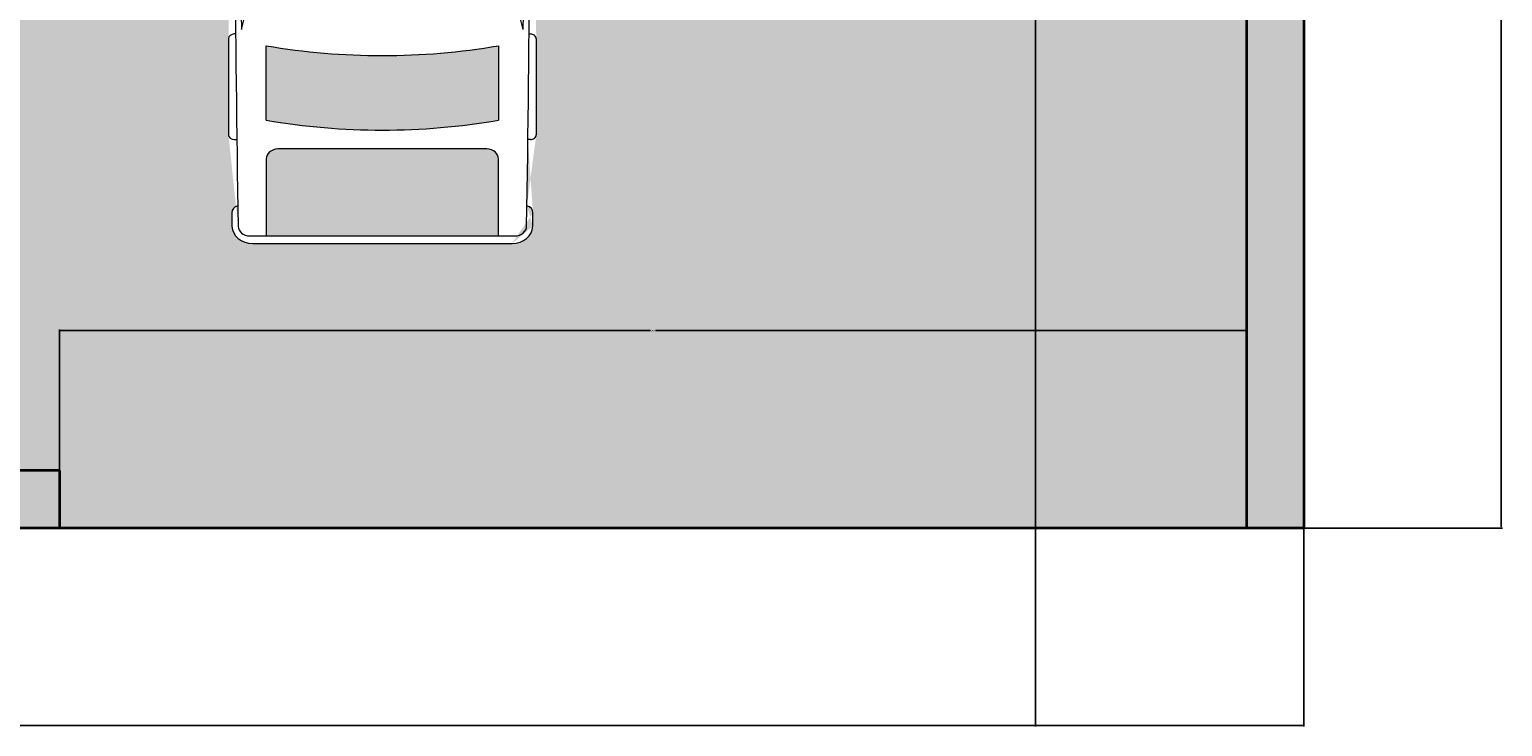
# Model space of a CAD drawing. Units: inches. Extents: x 2549 to 3108, y 1683 to 2362.
# Tile 4 of 30: x 2877 to 3108, y 1683 to 1793. Entities that reach past the tile are written whole.
import ezdxf

# ---------------------------------------------------------------- set-up
doc = ezdxf.new("R2010")
doc.units = ezdxf.units.IN
for name, color, linetype, lineweight in [('A-ANNO-DIMS', 2, 'Continuous', 18), ('C-PKNG-VEHI', 8, 'Continuous', 18), ('C-PROP', 7, 'Continuous', 35)]:
    doc.layers.add(name, color=color, linetype=linetype, lineweight=lineweight)
for name, color, linetype, lineweight, true_color in [('C-PKNG-VEHI-PATT', 251, 'Continuous', 13, 0x636466), ('C-PROP-PATT', 252, 'Continuous', 13, 0x939598), ('C-PVMT-PATT', 9, 'Continuous', 13, 0xc7c8ca)]:
    doc.layers.add(name, color=color, linetype=linetype, lineweight=lineweight, true_color=true_color)
doc.styles.get("Standard").update_dxf_attribs({"font": 'arial.ttf'})
doc.dimstyles.get("Standard").update_dxf_attribs({"dimtxt": 0.18, "dimasz": 0.18, "dimexe": 0.18, "dimexo": 0.0625, "dimgap": 0.09, "dimtad": 0, "dimtih": 1, "dimtoh": 1, "dimdec": 4, "dimzin": 0, "dimdsep": 46, "dimtxsty": 'Standard', "dimcen": 0.09, "dimadec": 0, "dimazin": 0, "dimtfac": 1, "dimtdec": 4, "dimtofl": 0, "dimtmove": 0, "dimatfit": 3, "dimfxl": 1, "dimtolj": 1, "dimtzin": 0, "dimarcsym": 0})

# ---------------------------------------------------------------- blocks, each defined once
blk = doc.blocks.new('*U11')
for p, q in [((21.10406751471477, 37.40863046792069), (21.10406751471477, 36.83230215753705)), ((46.55368679439944, 38.88847654282876), (22.35054758993934, 38.88847654282876)), ((47.80016686962392, 37.39011648242055), (47.80016686962392, 37.40863046792069)), ((135.4513231603356, 37.07354110333037), (135.4513231603356, 37.40863046792069)), ((136.6978032355602, 38.88847654282876), (160.90094244002, 38.88847654282867)), ((162.1474225152445, 37.40863046792049), (162.1474225152445, 36.77402019194128)), ((87.98532186932616, 31.87120872459877), (74.75900729854769, 35.92175679182955)), ((134.313356548143, 35.6043097713567), (119.2882629232503, 31.77757799177584)), ((70.0302824853563, 31.53613089391356), (86.40615155322342, 29.35124891408057)), ((186.4728846989705, -33.49860931502491), (186.4728846989718, 33.49860931502465)), ((188.3990091454065, -32.75868627757393), (188.3990091454077, 32.75868627757058)), ((138.4228833961707, 29.35124891408074), (157.2465674415997, 29.35124891408074)), ((164.515393597658, 26.39155676426461), (164.5153935976578, -26.39155676426503)), ((186.4728846989718, 29.35124891408083), (167.0083537481071, 29.35124891408083)), ((32.26591480791686, 11.62530558863241), (36.12873726252356, 17.16961494239206)), ((36.12873726252356, 17.16961494239206), (50.93891189819171, 17.16961494239206)), ((29.77279020470884, 9.505833383620029), (51.68362801571248, 9.505833383620029)), ((32.12291633764599, 9.505833383620029), (32.12291633764599, 11.15369945057711)), ((58.9167604809788, -10.77488335095668), (58.9167604809788, 10.77488335095617)), ((66.55009204259746, -10.5288681329018), (66.55009204259746, 10.52886813290129)), ((82.73706193978568, 8.496039918672748), (82.73706193978568, -8.49603991867258)), ((186.4728846989718, -10.5288681329018), (186.4728846989718, 10.52886813290129)), ((3.266462181856987, 6.128290093440767), (0.1022408397004821, 0.4060708604429806)), ((-4.43e-14, -2.558e-13), (51.68362801571248, -2.558e-13)), ((0.1022408397004821, -0.4060708604432933), (3.266462181856987, -6.128290093441194)), ((29.77279020470884, -9.50583338362054), (51.68362801571248, -9.50583338362054)), ((32.12291633764599, -9.50583338362054), (32.12291633764599, -11.15369945057762)), ((32.26591480791686, -11.62530558863292), (36.12873726252356, -17.16961494239257)), ((36.12873726252356, -17.16961494239257), (50.93891189819171, -17.16961494239257)), ((86.40615155322318, -29.35124891408145), (70.03028248535594, -31.53613089391442)), ((157.2465674415997, -29.35124891408117), (138.4228833961707, -29.35124891408126)), ((167.008353748107, -29.35124891408126), (186.4728846989707, -29.35124891408108)), ((87.98532186932607, -31.87120872459903), (74.7590072985476, -35.92175679182964)), ((134.3133565481428, -35.60430977135721), (119.2882629232503, -31.77757799177618)), ((21.10406751471477, -37.4086304679212), (21.10406751471477, -36.83230215753756)), ((135.4513231603355, -37.07354110333088), (135.4513231603355, -37.4086304679212)), ((162.1474225152445, -37.408630467921), (162.1474225152445, -36.77402019194179)), ((46.55368679439944, -38.88847654282927), (22.35054758993934, -38.88847654282927)), ((47.80016686962392, -37.39011648242107), (47.80016686962392, -37.4086304679212)), ((136.6978032355602, -38.88847654282927), (160.9009424400199, -38.88847654282918))]:
    blk.add_line(p, q)
for centre, major_axis, ratio, start_param, end_param in [((41.19115208863305, -490.8631038926156), (1.294e-13, 528.2339998381949), 0.8423038695439741, 0.0028100083536837, 0.0755983031096952), ((22.35054758993934, 37.40863046792072), (2.08e-14, -1.479846074908118), 0.842303869543976, 3.141592653589776, 4.712388980384677), ((64.48199294511879, -10555.61767587835), (1.907644e-10, 10593.02630634627), 0.842303869543847, -0.0133969486112073, 0.0027970409639888), ((46.55368679439944, 37.40863046792072), (2.2e-14, 1.479846074908118), 0.8423038695439758, -1.570796326794884, 1.73e-14), ((136.6978032355602, 37.40863046792072), (2.357e-13, -1.479846074908118), 0.842303869543976, 3.141592653589603, 4.712388980384554), ((160.90094244002, 37.40863046792052), (5.59e-14, 1.479846074908118), 0.842303869543976, -1.570796326794865, 4.44e-14), ((180.6280394947615, 35.8381667808375), (7.4e-14, 2.219769112362114), 0.8423038695439693, -0.0130174256259048, 1.249894140392862), ((64.48199294754608, -10556.35759891604), (1.349839377e-06, 10595.3130398087), 0.8423038681351469, -0.0133969484821159, -0.0130174254969711), ((183.9799245485216, 32.75868627756583), (8.56e-14, -5.246425615115243), 0.8423038695439737, 1.570796326795794, 3.128195704978164), ((266.0300214172791, -27.52442688366631), (1.966072e-10, 313.3077612809058), 0.8423038695435284, 1.367075990158062, 1.391760499156098), ((64.4819929449925, -10555.61767590795), (1.9177683e-09, -10591.54646030096), 0.8423038695482963, 3.133765086725325, 3.140440689641252), ((183.9799245485226, 33.49860931502124), (3e-16, -2.959692149816168), 0.8423038695439952, 1.570796326796048, 3.128195704978389), ((135.2911776514449, 5.387441675478555), (2.2715e-12, 81.77258453065997), 0.8423038695439563, 1.245306111696802, 1.507880129813836), ((95.78879860270445, -3666.353346297651), (1.949864e-10, -3698.236159209632), 0.8423038695446962, 3.134048706297306, 3.14409775411291), ((259.1750197310735, -27.52442688366614), (1.506617e-10, -305.3028914627677), 0.8423038695443789, 4.528606069860317, 4.561837674556238), ((37.47375371777758, -593.9621830607928), (6.21e-14, -623.32820996736), 0.8423038695439826, 3.09604606856106, 3.200911180495224), ((134.4003789125686, 5.387441675477674), (4.276e-13, -89.7774543484738), 0.84230386954398, 4.44948196380473, 4.652344057257214), ((149.595361812917, 2.799442537139299), (8.561e-13, -79.57966406425402), 0.842303869543983, 4.372215489277867, 4.640744122441986), ((17.08207736189386, -1.421e-13), (6.87e-14, 147.0179238898305), 0.8423038695439764, 4.511394369635731, 4.913383591133647), ((35.90576140732288, -1.421e-13), (6.87e-14, 147.0179238898305), 0.8423038695439764, 4.511394369635731, 4.913383591133647), ((167.0083537481071, 26.39155676426464), (1.394e-13, 2.959692149816236), 0.842303869543976, 5.55e-14, 1.57079632679492), ((-204.4946649195746, 52.39684969293512), (4.12053e-11, -250.9602162198571), 0.8423038695441164, 1.385369446298923, 1.434372047871027), ((13.03653510440275, 17.00972444508943), (1.2303e-12, 27.41599049210566), 0.8423038695439277, 4.435146050259648, 4.718221029521873), ((14.20086229321332, 17.00972444508943), (1.2303e-12, 27.41599049210566), 0.8423038695439277, 4.435146050259648, 4.718221029521873), ((50.7902773840875, 13.33772416300607), (6.340077547122382, -0.356608581037027), 0.6038335755719145, -1.39555193967809, 1.581314658479915), ((32.74615637525823, 11.15369945057713), (1.313e-13, 0.7399230374541176), 0.8423038695439091, 0.8797135699495516, 1.570796326795045), ((29.77279020470884, -46.66302566589627), (5.12e-14, 56.16885904951626), 0.842303869543976, 7e-16, 0.5903187773915901), ((0.6232400376122422, -1.421e-13), (1e-16, -0.7399230374541245), 0.842303869543842, 4.131459131953847, 5.293318828815531), ((29.77279020470884, 46.66302566589578), (4.004e-13, 56.16885904951626), 0.8423038695439734, 2.55127387619821, 3.141592653589801), ((-204.4946649195746, -52.39684969293552), (4.02945e-11, 250.9602162198562), 0.8423038695441192, -1.43437204787103, -1.385369446298926), ((32.74615637525823, -11.1536994505777), (1.3e-13, -0.7399230374541176), 0.8423038695439093, 4.712388980384541, 5.403471737230034), ((13.03653510440275, -17.00972444508983), (1.2568e-12, -27.41599049210552), 0.8423038695439318, 1.564964277657711, 1.848039256919935), ((14.20086229321332, -17.00972444508983), (1.2568e-12, -27.41599049210552), 0.8423038695439318, 1.564964277657711, 1.848039256919935), ((134.4003789125684, -5.387441675478584), (4.2949e-12, -89.77745434847827), 0.8423038695439354, -1.510751403667474, -1.307889310215002), ((135.2911776514465, -5.387441675480715), (3.2038e-12, -81.77258453066244), 0.8423038695439492, -1.50788012981387, -1.245306111696839), ((149.5953618129329, -2.799442537137565), (4.0897e-12, -79.57966406427697), 0.8423038695439419, -1.499151468852248, -1.230622835688196), ((259.1750197310694, 27.52442688365929), (1.08535e-11, 305.3028914629043), 0.8423038695439974, 1.721347632622872, 1.754579237318777), ((266.0300214172791, 27.52442688366566), (8.75241e-11, 313.3077612806533), 0.8423038695441819, 1.749832154434603, 1.774516663432659), ((37.47375371777847, 593.9621830607904), (1.1693e-12, -623.3282099673584), 0.8423038695439528, -0.0593185269054384, 0.0455465850287298), ((167.008353748107, -26.39155676426503), (1.02e-14, -2.959692149816192), 0.8423038695439885, 4.712388980384686, 6.283185307179581), ((95.78879860271888, 3666.35334629765), (1.637818e-10, -3698.236159209629), 0.8423038695447546, -0.0025051005232382, 0.007543947292366), ((183.9799245485216, -33.4986093150211), (9.3e-15, 2.959692149816141), 0.8423038695439732, 3.154989602201626, 4.71238898038339), ((183.9799245485177, -32.7586862775633), (2.428e-13, -5.246425615118353), 0.8423038695439808, 0.0133969486110846, 1.570796326792831), ((41.19115208863322, 490.8631038926152), (1.37757e-11, -528.2339998381949), 0.8423038695440652, -0.0755983031097181, -0.0028100083537155), ((64.48199294495228, 10555.61767590795), (6.117947e-10, 10593.02630637587), 0.8423038695458146, 3.138795612625926, 3.154989602201039), ((64.48199294503607, 10555.61767590793), (1.6049794e-09, -10591.54646030094), 0.8423038695397146, 0.0011519639481523, 0.0078275668641468), ((180.6280394947581, -35.83816678083949), (2.274e-13, -2.219769112363032), 0.8423038695439803, -1.249894138785958, 0.0130174256254374), ((22.35054758993934, -37.40863046792117), (2.2e-14, 1.479846074908118), 0.8423038695439758, 1.570796326794908, 3.14159265358981), ((46.55368679439944, -37.40863046792117), (2.08e-14, -1.479846074908118), 0.842303869543976, -1.69e-14, 1.570796326794884), ((136.6978032355602, -37.40863046792109), (1.56e-14, -1.479846074908162), 0.8423038695440105, -1.570796326794875, -1.27e-14), ((160.9009424400199, -37.408630467921), (1.969e-13, 1.479846074908162), 0.8423038695440109, 3.141592653589951, 4.712388980384771), ((64.48199294197605, 10556.3575989598), (9.365289701e-07, 10595.31303985772), 0.8423038705260315, 3.154610079306566, 3.154989602290631)]:
    blk.add_ellipse(centre, major_axis=major_axis, ratio=ratio, start_param=start_param, end_param=end_param)
at = {"extrusion": (0, 0, -1)}
blk.add_ellipse((50.7902773840875, -13.33772416300655), major_axis=(6.340077547122382, 0.3566085810370246), ratio=0.6038335755719145, start_param=-1.39555193967809, end_param=1.581314658479915, dxfattribs=at)
blk = doc.blocks.new('*D24')
at = {"layer": 'A-ANNO-DIMS', "color": 0, "lineweight": -2, "transparency": 16777216}
for p, q in [((2596.642666000001, 1714.461244), (2596.642666000001, 1683.443744)), ((3076.642666000001, 1714.461244), (3076.642666000001, 1683.443744)), ((2596.822666, 1683.623744), (2836.350503653479, 1683.623744)), ((3076.462666000001, 1683.623744), (2836.934828346521, 1683.623744))]:
    blk.add_line(p, q, dxfattribs=at)
at = {"layer": 'A-ANNO-DIMS', "color": 0, "transparency": 16777216}
for points in [[(2596.822666, 1683.653744), (2596.822666, 1683.593744), (2596.642666000001, 1683.623744)], [(3076.462666000001, 1683.653744), (3076.462666000001, 1683.593744), (3076.642666000001, 1683.623744)]]:
    blk.add_solid(points, dxfattribs=at)
at = {"layer": 'Defpoints', "color": 0, "transparency": 16777216}
for p in [(2596.642666000001, 1714.523744), (3076.642666000001, 1714.523744), (3076.642666000001, 1683.623744)]:
    blk.add_point(p, dxfattribs=at)
at = {"layer": 'A-ANNO-DIMS', "color": 0, "transparency": 16777216, "insert": (2836.642666, 1683.623744), "char_height": 0.18, "attachment_point": 5}
blk.add_mtext('\\A1;480', dxfattribs=at)
blk = doc.blocks.new('*D25')
at = {"layer": 'A-ANNO-DIMS', "color": 0, "lineweight": -2, "transparency": 16777216}
for p, q in [((3076.705166000002, 2314.523744000001), (3107.722666000003, 2314.523744000001)), ((3107.542666000004, 2314.343744000001), (3107.542666000004, 2014.705647137791)), ((3107.542666000004, 1714.703744000001), (3107.542666000004, 2014.341840862211)), ((3076.705166000002, 1714.523744000001), (3107.722666000003, 1714.523744000001))]:
    blk.add_line(p, q, dxfattribs=at)
at = {"layer": 'A-ANNO-DIMS', "color": 0, "transparency": 16777216}
for points in [[(3107.512666000003, 2314.343744000001), (3107.572666000004, 2314.343744000001), (3107.542666000004, 2314.523744000001)], [(3107.512666000003, 1714.703744000001), (3107.572666000004, 1714.703744000001), (3107.542666000004, 1714.523744000001)]]:
    blk.add_solid(points, dxfattribs=at)
at = {"layer": 'Defpoints', "color": 0, "transparency": 16777216}
for p in [(3076.642666000002, 2314.523744000001), (3107.542666000004, 2314.523744000001), (3076.642666000002, 1714.523744000001)]:
    blk.add_point(p, dxfattribs=at)
at = {"layer": 'A-ANNO-DIMS', "color": 0, "transparency": 16777216, "insert": (3107.542666000003, 2014.523743999999), "char_height": 0.18, "attachment_point": 5}
blk.add_mtext('\\A1;600', dxfattribs=at)
blk = doc.blocks.new('*D46')
at = {"layer": 'A-ANNO-DIMS', "color": 0, "lineweight": -2, "transparency": 16777216}
for p, q in [((2812.642666, 2140.461244), (2812.642666, 1683.443744)), ((3034.642666, 2134.461244), (3034.642666, 1683.443744)), ((2812.822666, 1683.623744), (2923.35320488131, 1683.623744)), ((3034.462666, 1683.623744), (2923.932127118691, 1683.623744))]:
    blk.add_line(p, q, dxfattribs=at)
at = {"layer": 'A-ANNO-DIMS', "color": 0, "transparency": 16777216}
for points in [[(2812.822666, 1683.653744), (2812.822666, 1683.593744), (2812.642666, 1683.623744)], [(3034.462666, 1683.653744), (3034.462666, 1683.593744), (3034.642666, 1683.623744)]]:
    blk.add_solid(points, dxfattribs=at)
at = {"layer": 'Defpoints', "color": 0, "transparency": 16777216}
for p in [(2812.642666, 2140.523744), (3034.642666, 2134.523744), (3034.642666, 1683.623744)]:
    blk.add_point(p, dxfattribs=at)
at = {"layer": 'A-ANNO-DIMS', "color": 0, "transparency": 16777216, "insert": (2923.642666000001, 1683.623744), "char_height": 0.18, "attachment_point": 5}
blk.add_mtext('\\A1;222', dxfattribs=at)
blk = doc.blocks.new('*D61')
at = {"layer": 'A-ANNO-DIMS', "color": 0, "lineweight": -2, "transparency": 16777216}
for p, q in [((2881.839988, 1714.586244), (2881.839988, 1745.603744)), ((2882.019988, 1745.423744), (2974.355910901774, 1745.423744)), ((3067.462666000001, 1745.423744), (2975.126743098227, 1745.423744)), ((3067.642666000001, 1714.586244), (3067.642666000001, 1745.603744))]:
    blk.add_line(p, q, dxfattribs=at)
at = {"layer": 'A-ANNO-DIMS', "color": 0, "transparency": 16777216}
for points in [[(2882.019988, 1745.453744), (2882.019988, 1745.393744), (2881.839988, 1745.423744)], [(3067.462666000001, 1745.453744), (3067.462666000001, 1745.393744), (3067.642666000001, 1745.423744)]]:
    blk.add_solid(points, dxfattribs=at)
at = {"layer": 'Defpoints', "color": 0, "transparency": 16777216}
for p in [(3067.642666000001, 1745.423744), (2881.839988, 1714.523744), (3067.642666000001, 1714.523744)]:
    blk.add_point(p, dxfattribs=at)
at = {"layer": 'A-ANNO-DIMS', "color": 0, "transparency": 16777216, "insert": (2974.741327, 1745.423744), "char_height": 0.18, "attachment_point": 5}
blk.add_mtext('\\A1;185.8', dxfattribs=at)

msp = doc.modelspace()

# ---------------------------------------------------------------- hatches: boundary and pattern name
at = {"layer": 'C-PKNG-VEHI-PATT'}
h = msp.add_hatch(color=256, dxfattribs=at)
h.dxf.hatch_style = 1
edge = h.paths.add_edge_path()
edge.add_ellipse((2935.725796552836, 1791.96404850691), major_axis=(-50.6600031146233, 6.78e-13), ratio=0.8423038695439883, start_angle=248.1650462032912, end_angle=265.7225790369452)
edge.add_line((2938.911028887629, 1834.550737322417), (2925.865275339109, 1834.550737322417))
edge.add_ellipse((2929.050507673901, 1791.964048506909), major_axis=(50.66000311462998, 7.2698e-12), ratio=0.8423038695438956, start_angle=94.27742096304536, end_angle=111.8349537966996)
edge.add_line((2912.850791291541, 1832.394679033669), (2914.204376096751, 1822.249450253823))
edge.add_ellipse((2930.653832861207, 1783.102276333115), major_axis=(-49.30143828149606, 1.1087e-12), ratio=0.8423038695440098, start_angle=-85.12993040286318, end_angle=-67.20808512241217, ccw=False)
edge.add_line((2927.124659327709, 1824.522535937876), (2937.65164489903, 1824.522535937876))
edge.add_ellipse((2934.122471365533, 1783.102276333124), major_axis=(49.30143828148681, 7.803e-13), ratio=0.8423038695439693, start_angle=67.20808512240922, end_angle=85.12993040286312, ccw=False)
edge.add_line((2950.571928129987, 1822.249450253823), (2951.925512935197, 1832.394679033669))
edge = h.paths.add_edge_path()
edge.add_ellipse((2903.479330909537, 1857.335124490177), major_axis=(-34.79790434319148, 3.2087e-12), ratio=0.8423038695440206, start_angle=180.0000000000052, end_angle=209.4385695979841)
edge.add_ellipse((2961.296973317201, 1857.335124490177), major_axis=(34.79790434319149, 1.2616e-12), ratio=0.8423038695439669, start_angle=150.5614304020187, end_angle=179.9999999999979)
edge.add_line((2926.49906897401, 1857.335124490177), (2926.49906897401, 1843.76085484809))
edge.add_ellipse((2924.125124210826, 1844.314306179491), major_axis=(-0.2209272451118966, 3.927824345135514), ratio=0.6038335755719296, start_angle=89.00201427502537, end_angle=253.65740804569998, ccw=False)
edge.add_line((2921.751179447642, 1844.222223668088), (2921.751179447642, 1853.39746861696))
edge.add_line((2921.751179447642, 1853.39746861696), (2925.26903797625, 1855.848425453852))
edge.add_ellipse((2925.478177919096, 1855.493055533625), major_axis=(0.4583993962922678, 2.303e-12), ratio=0.8423038695418179, start_angle=89.9999999997122, end_angle=134.4802108822853, ccw=False)
edge.add_line((2925.478177919095, 1855.879167118917), (2926.49906897401, 1855.879167118917))
edge.add_line((2926.49906897401, 1855.879167118917), (2926.49906897401, 1857.335124490177))
edge.add_ellipse((2961.296973317201, 1857.335124490177), major_axis=(34.79790434319149, 1.2616e-12), ratio=0.8423038695439669, start_angle=150.5614304020187, end_angle=179.999999999998, ccw=False)
edge.add_line((2932.388152113369, 1873.650056952746), (2932.388152113369, 1875.780055063896))
edge.add_ellipse((2932.388152113369, 1875.393943478604), major_axis=(0.4583993962904624, 1e-16), ratio=0.8423038695446395, start_angle=89.99999999999999, end_angle=127.9331304598429)
edge.add_line((2932.136581844764, 1875.716714504374), (2928.591534983032, 1873.756406364807))
edge.add_ellipse((2899.927094610101, 2002.469218934773), major_axis=(155.4756451483881, 9.82606e-11), ratio=0.842303869543439, start_angle=-80.74343399283458, end_angle=-77.44506735589891, ccw=False)
edge.add_ellipse((2949.440169726089, 1715.215149574257), major_axis=(-189.1421864819335, 9.35831e-11), ratio=0.8423038695443681, start_angle=-79.79046100282835, end_angle=-77.55537270652765)
edge.add_ellipse((3300.361430890526, 1852.564199885104), major_axis=(-386.1662101011402, 3.282e-12), ratio=0.8423038695438535, start_angle=-2.863714607837213, end_angle=2.198540565955553)
edge.add_ellipse((2929.050507673902, 1792.515918881865), major_axis=(-55.61920468847034, 9.624e-12), ratio=0.842303869544118, start_angle=-85.91758930883981, end_angle=-72.28004677724027, ccw=False)
edge.add_line((2925.712863234435, 1839.27976237288), (2939.063440992303, 1839.27976237288))
edge.add_ellipse((2935.725796552836, 1792.515918881865), major_axis=(55.61920468846977, 1.19088e-11), ratio=0.8423038695441256, start_angle=72.28004677723749, end_angle=85.91758930883759, ccw=False)
edge.add_ellipse((2564.414873336211, 1852.564199885105), major_axis=(-386.166210101141, 7.3121e-12), ratio=0.8423038695442235, start_angle=177.8014594340458, end_angle=182.8637146078386)
edge.add_ellipse((2915.336134500645, 1715.215149574254), major_axis=(189.1421864814668, 5.425418e-10), ratio=0.8423038695464061, start_angle=77.5553727063904, end_angle=79.79046100269107)
edge.add_ellipse((2964.849209616638, 2002.469218934773), major_axis=(-155.4756451483861, 9.70869e-11), ratio=0.8423038695434499, start_angle=77.44506735589852, end_angle=80.74343399283418, ccw=False)
edge.add_line((2936.184769243706, 1873.756406364807), (2932.639722381973, 1875.716714504375))
edge.add_ellipse((2932.388152113369, 1875.393943478604), major_axis=(0.4583993962904624, 1e-16), ratio=0.8423038695446395, start_angle=52.06686954015704, end_angle=89.99999999999999)
edge.add_line((2932.388152113369, 1875.780055063896), (2932.388152113369, 1873.650056952746))
edge.add_ellipse((2903.479330909537, 1857.335124490177), major_axis=(-34.79790434319148, 3.2087e-12), ratio=0.8423038695440206, start_angle=180.0000000000053, end_angle=209.4385695979841, ccw=False)
edge.add_line((2938.277235252728, 1857.335124490177), (2938.277235252728, 1855.879167118917))
edge.add_line((2938.277235252728, 1855.879167118917), (2939.405880844674, 1855.879167118917))
edge.add_ellipse((2939.298126307642, 1855.493055533625), major_axis=(-0.4583993962922676, 2.3028e-12), ratio=0.8423038695418185, start_angle=225.5197891177147, end_angle=270.00000000028786, ccw=False)
edge.add_line((2939.590297193029, 1855.790576266728), (2943.025124779096, 1853.39746861696))
edge.add_line((2943.025124779096, 1853.39746861696), (2943.025124779096, 1844.222223668088))
edge.add_ellipse((2940.651180015912, 1844.314306179491), major_axis=(0.2209272451118966, 3.927824345135514), ratio=0.6038335755719296, start_angle=106.3425919543001, end_angle=270.9979857249746, ccw=False)
edge.add_line((2938.277235252728, 1843.76085484809), (2938.277235252728, 1857.335124490177))
edge = h.paths.add_edge_path()
edge.add_ellipse((2932.388152113369, 1865.19731394932), major_axis=(91.08099646002908, 7.134e-13), ratio=0.8423038695439837, start_angle=256.4018653097688, end_angle=283.5981346902299, ccw=False)
edge.add_line((2914.204376096751, 1790.023884530285), (2914.204376096751, 1778.36217788565))
edge.add_ellipse((2932.388152113369, 1853.535607304685), major_axis=(91.08099646002908, 7.134e-13), ratio=0.8423038695439837, start_angle=256.4018653097688, end_angle=283.5981346902299)
edge.add_line((2950.571928129987, 1778.36217788565), (2950.571928129987, 1790.023884530285))
edge = h.paths.add_edge_path()
edge.add_ellipse((2948.738330544823, 1772.31452600415), major_axis=(1.833597585163715, 1.1861e-12), ratio=0.8423038695440299, start_angle=-3.70558e-11, end_angle=89.99999999996297)
edge.add_line((2948.738330544824, 1773.85897234532), (2916.037973681915, 1773.858972345321))
edge.add_ellipse((2916.037973681915, 1772.314526004151), major_axis=(1.833597585163716, 6.788e-13), ratio=0.84230386954403, start_angle=89.9999999999788, end_angle=179.9999999999787)
edge.add_line((2914.204376096751, 1772.314526004151), (2914.204376096751, 1760.255799913309))
edge.add_line((2914.204376096751, 1760.255799913309), (2950.571928129987, 1760.255799913308))
edge.add_line((2950.571928129987, 1760.255799913308), (2950.571928129987, 1772.31452600415))
h.paths.add_polyline_path([(2748.849609196547, 2101.638310911291), (2798.147998217048, 2101.638310911291), (2798.147998217048, 2111.424826549233), (2748.849609196547, 2111.424826549233)], flags=9)
h.paths.add_polyline_path([(2685.208067619545, 2101.488974631509), (2719.325307162104, 2101.488974631509), (2719.325307162104, 2111.281945754699), (2685.208067619545, 2111.281945754699)], flags=9)
h.paths.add_polyline_path([(2814.685179139321, 1907.132804880864), (2847.838399551318, 1907.132804880864), (2847.838399551318, 1916.925776004054), (2814.685179139321, 1916.925776004054)], flags=9)
h.paths.add_polyline_path([(2814.390575309562, 1835.586397562281), (2848.017197973174, 1835.586397562281), (2848.017197973174, 1845.379368685471), (2814.390575309562, 1845.379368685471)], flags=9)
h.paths.add_polyline_path([(2800.524456569608, 1759.167447237475), (2853.743476964851, 1759.167447237475), (2853.743476964851, 1768.953962875417), (2800.524456569608, 1768.953962875417)], flags=9)
h.paths.add_polyline_path([(2972.461062245805, 1807.33049128039), (3015.394342810494, 1807.33049128039), (3015.394342810494, 1817.117006918332), (2972.461062245805, 1817.117006918332)], flags=9)
h.paths.add_polyline_path([(2902.332650472062, 1888.673085326325), (2937.913133337796, 1888.673085326325), (2937.913133337796, 1898.466056449515), (2902.332650472062, 1898.466056449515)], flags=9)
h.paths.add_polyline_path([(2712.17793111998, 1878.903902566108), (2754.125674269943, 1878.903902566108), (2754.125674269943, 1888.69041820405), (2712.17793111998, 1888.69041820405)], flags=9)
h.paths.add_polyline_path([(2614.005606808349, 2012.811964980989), (2650.025062671036, 2012.811964980989), (2650.025062671036, 2022.437093487698), (2614.005606808349, 2022.437093487698)], flags=9)
h.paths.add_polyline_path([(2713.312922761346, 2003.164487508756), (2747.423706818656, 2003.164487508756), (2747.423706818656, 2012.951003146698), (2713.312922761346, 2012.951003146698)], flags=9)
h.paths.add_polyline_path([(2950.137937233872, 2001.693439459313), (2982.299164745893, 2001.693439459313), (2982.299164745893, 2011.479955097255), (2950.137937233872, 2011.479955097255)], flags=9)
h.paths.add_polyline_path([(2940.863994744806, 2238.553674899427), (2997.506574150595, 2238.553674899427), (2997.506574150595, 2248.346646022617), (2940.863994744806, 2248.346646022617)], flags=9)
h.paths.add_polyline_path([(2821.545730132573, 2202.834824551463), (2855.662969675132, 2202.834824551463), (2855.662969675132, 2212.627795674654), (2821.545730132573, 2212.627795674654)], flags=9)
h.paths.add_polyline_path([(2661.802564922812, 2238.624912952816), (2718.445144328601, 2238.624912952816), (2718.445144328601, 2248.417884076006), (2661.802564922812, 2248.417884076006)], flags=9)
at = {"layer": 'C-PROP-PATT'}
h = msp.add_hatch(color=256, dxfattribs=at)
h.dxf.hatch_style = 1
h.paths.add_polyline_path([(3076.642666391656, 2314.523744486262), (2596.642666391656, 2314.523744486262), (2596.642666391656, 1714.523744486262), (2881.839988255281, 1714.523744486262), (2881.839988255281, 1723.523744486262), (2605.642666391656, 1723.523744486262), (2605.642666391656, 2305.523744486262), (3067.642666391656, 2305.523744486262), (3067.642666391656, 1723.523744486262), (3067.642666391656, 1714.523744486262), (3076.642666391656, 1714.523744486262)])
at = {"layer": 'C-PVMT-PATT'}
h = msp.add_hatch(color=256, dxfattribs=at)
h.dxf.hatch_style = 1
h.paths.add_polyline_path([(3067.642666391656, 2305.523744486262), (2605.642666391656, 2305.523744486262), (2605.642666391656, 2074.523744486262), (2629.642666391656, 2074.523744486262), (2629.642666391656, 2281.523744486262), (3043.642666391656, 2281.523744486262), (3043.642666391656, 1885.523744486263), (3043.642666391656, 1872.874514030248), (3031.167181590035, 1872.874514030248), (3031.167181590035, 1862.573058982011), (2995.805391311171, 1862.573058982011), (2995.805391311171, 1872.874514030248), (2983.175155144805, 1872.874514030248), (2983.175155144805, 1885.523744486262), (2881.642666391656, 1885.523744486263), (2881.642666391656, 1795.523744486262), (2751.09773888662, 1795.523744486262), (2751.09773888662, 1761.523744486262), (2786.157685455576, 1761.523744486262), (2786.157685455577, 1723.523744486262), (2881.839988255281, 1723.523744486262), (2881.839988255281, 1714.523744486262), (3067.642666391656, 1714.523744486262), (3067.642666391656, 1723.523744486262)])
edge = h.paths.add_edge_path(flags=16)
edge.add_ellipse((2949.440169726093, 1710.96831784248), major_axis=(-194.1013880556022, 3.100242e-10), ratio=0.8423038695451509, start_angle=-77.87403444762441, end_angle=-76.21947101041059, ccw=False)
edge.add_ellipse((2949.440169726089, 1715.215149574257), major_axis=(-189.1421864819335, 9.35831e-11), ratio=0.8423038695443681, start_angle=-79.7904610028283, end_angle=-77.55537270652758, ccw=False)
edge.add_ellipse((2899.927094610101, 2002.469218934773), major_axis=(155.4756451483881, 9.82606e-11), ratio=0.842303869543439, start_angle=-80.74343399283462, end_angle=-77.44506735589897)
edge.add_line((2928.591534983032, 1873.756406364807), (2932.388152113369, 1875.855825569603))
edge.add_line((2932.388152113369, 1875.855825569603), (2936.184769243706, 1873.756406364807))
edge.add_ellipse((2964.849209616638, 2002.469218934773), major_axis=(-155.4756451483861, 9.70869e-11), ratio=0.8423038695434499, start_angle=77.4450673558985, end_angle=80.74343399283416)
edge.add_ellipse((2915.336134500645, 1715.215149574254), major_axis=(189.1421864814668, 5.425418e-10), ratio=0.8423038695464061, start_angle=77.55537270639041, end_angle=79.79046100269102, ccw=False)
edge.add_ellipse((2915.336134500645, 1710.96831784248), major_axis=(-194.1013880561466, 2.794238e-10), ratio=0.8423038695428703, start_angle=256.2194710105847, end_angle=257.8740344477983, ccw=False)
edge.add_ellipse((2628.287132012546, 1850.261185811051), major_axis=(-327.2531525161749, 1.24457e-11), ratio=0.8423038695440036, start_angle=182.1799503136474, end_angle=183.6504275857012, ccw=False)
edge.add_ellipse((2955.563661936079, 1861.933375066942), major_axis=(-0.9167987925820851, 6.203e-13), ratio=0.8423038695438211, start_angle=180.0000000000388, end_angle=270.00000000003877, ccw=False)
edge.add_line((2956.480460728661, 1862.385732927092), (2956.480460728661, 1846.486613953928))
edge.add_ellipse((2955.563661936079, 1846.938971814078), major_axis=(-0.9167987925816303, 6.983e-13), ratio=0.8423038695442389, start_angle=90.0000000000436, end_angle=180.0000000000437, ccw=False)
edge.add_ellipse((-3607.060581297885, 1835.831972437108), major_axis=(-6562.624243233964, 2.000376e-10), ratio=0.8423038695434055, start_angle=179.6161332212093, end_angle=180.0902290885961, ccw=False)
edge.add_ellipse((2955.563661936079, 1791.092611498023), major_axis=(0.9167987925816303, 1.8053e-12), ratio=0.8423038695442389, start_angle=-1.127773430198431e-10, end_angle=89.99999999988711, ccw=False)
edge.add_line((2956.480460728661, 1791.544969358173), (2956.480460728661, 1775.645850385008))
edge.add_ellipse((2955.563661936079, 1776.098208245159), major_axis=(0.9167987925816303, 5.91e-14), ratio=0.8423038695442391, start_angle=269.9999999999963, end_angle=359.9999999999963, ccw=False)
edge.add_ellipse((-3607.060581297885, 1835.831972437108), major_axis=(-6562.624243233964, 2.000376e-10), ratio=0.8423038695434055, start_angle=179.3813568036826, end_angle=179.4717285281838, ccw=False)
edge.add_ellipse((2954.590723441648, 1763.876816393945), major_axis=(-1.375198188872997, 3.586e-13), ratio=0.8423038695436877, start_angle=179.3717627838213, end_angle=248.4647566010281, ccw=False)
edge.add_ellipse((-3607.518980694323, 1835.831972435604), major_axis=(-6564.040927375597, 4.0829067806e-06), ratio=0.8423038626957529, start_angle=179.3534459385899, end_angle=179.371762819423, ccw=False)
edge.add_ellipse((2952.682914207262, 1761.800246254478), major_axis=(3.250281735962, 3.921e-13), ratio=0.8423038695438826, start_angle=-89.99999999994031, end_angle=-0.6465540970884831, ccw=False)
edge.add_line((2952.682914207266, 1759.06252137117), (2912.093390019471, 1759.062521371171))
edge.add_ellipse((2912.093390019478, 1761.800246254481), major_axis=(3.250281735963338, 1.2841e-12), ratio=0.8423038695440954, start_angle=180.6465540970387, end_angle=269.99999999984414, ccw=False)
edge.add_ellipse((9472.295284948175, 1835.831972439052), major_axis=(-6564.040927413921, 8.323842912e-07), ratio=0.8423038709559154, start_angle=0.6282372235086768, end_angle=0.646554104341817, ccw=False)
edge.add_ellipse((2910.185580785089, 1763.876816393947), major_axis=(1.375198188873441, 9.687e-13), ratio=0.8423038695438604, start_angle=111.53524350397811, end_angle=180.6282372161342, ccw=False)
edge.add_ellipse((9471.836885542962, 1835.831972437208), major_axis=(-6562.624243252301, 3.836442e-10), ratio=0.8423038695462286, start_angle=0.5282714718206876, end_angle=0.6465540970643247, ccw=False)
edge.add_ellipse((2909.212642290659, 1776.098208245159), major_axis=(-0.9167987925820851, 6.203e-13), ratio=0.8423038695438211, start_angle=3.8824055081931874e-11, end_angle=90.00000000003882, ccw=False)
edge.add_line((2908.295843498077, 1775.645850385009), (2908.295843498077, 1791.544969358173))
edge.add_ellipse((2909.212642290659, 1791.092611498023), major_axis=(-0.9167987925820851, 4.868e-13), ratio=0.8423038695438213, start_angle=-89.99999999996948, end_angle=3.041122909053229e-11, ccw=False)
edge.add_ellipse((9471.836885542962, 1835.831972437208), major_axis=(-6562.624243252301, 3.836442e-10), ratio=0.8423038695462286, start_angle=-0.09022908858980827, end_angle=0.38386677879560693, ccw=False)
edge.add_ellipse((2909.212642290658, 1846.938971814078), major_axis=(-0.9167987925816306, 1.1661e-12), ratio=0.8423038695442389, start_angle=7.287326297955588e-11, end_angle=90.00000000007287, ccw=False)
edge.add_line((2908.295843498077, 1846.486613953928), (2908.295843498077, 1862.385732927092))
edge.add_ellipse((2909.212642290658, 1861.933375066942), major_axis=(0.9167987925816303, 1.1659e-12), ratio=0.8423038695442391, start_angle=89.99999999992713, end_angle=179.9999999999272, ccw=False)
edge.add_ellipse((3236.489172214191, 1850.261185811051), major_axis=(327.2531525161745, 3.33005e-11), ratio=0.8423038695444386, start_angle=176.3495724142951, end_angle=177.820049686349, ccw=False)
edge = h.paths.add_edge_path(flags=0)
edge.add_ellipse((2903.479330909537, 1857.335124490177), major_axis=(-34.79790434319148, 3.2087e-12), ratio=0.8423038695440206, start_angle=180.0000000000053, end_angle=209.4385695979841, ccw=False)
edge.add_line((2938.277235252728, 1857.335124490177), (2938.277235252728, 1855.879167118917))
edge.add_line((2938.277235252728, 1855.879167118917), (2939.463142736354, 1855.879167118917))
edge.add_line((2939.463142736354, 1855.879167118917), (2943.025124779096, 1853.39746861696))
edge.add_line((2943.025124779096, 1853.39746861696), (2943.025124779096, 1844.222223668088))
edge.add_ellipse((2940.651180015912, 1844.314306179491), major_axis=(0.2209272451118966, 3.927824345135514), ratio=0.6038335755719296, start_angle=106.3425919543001, end_angle=270.9979857249746, ccw=False)
edge.add_line((2938.277235252728, 1843.76085484809), (2938.277235252728, 1857.335124490177))
edge.add_ellipse((2903.479330909537, 1857.335124490177), major_axis=(-34.79790434319148, 3.2087e-12), ratio=0.8423038695440206, start_angle=180.0000000000052, end_angle=209.4385695979841)
edge.add_ellipse((2961.296973317201, 1857.335124490177), major_axis=(34.79790434319149, 1.2616e-12), ratio=0.8423038695439669, start_angle=150.5614304020187, end_angle=179.9999999999979)
edge.add_line((2926.49906897401, 1857.335124490177), (2926.49906897401, 1843.76085484809))
edge.add_ellipse((2924.125124210826, 1844.314306179491), major_axis=(-0.2209272451118966, 3.927824345135514), ratio=0.6038335755719296, start_angle=89.00201427502537, end_angle=253.65740804569998, ccw=False)
edge.add_line((2921.751179447642, 1844.222223668088), (2921.751179447642, 1853.39746861696))
edge.add_line((2921.751179447642, 1853.39746861696), (2925.313161490385, 1855.879167118917))
edge.add_line((2925.313161490385, 1855.879167118917), (2926.49906897401, 1855.879167118917))
edge.add_line((2926.49906897401, 1855.879167118917), (2926.49906897401, 1857.335124490177))
edge.add_ellipse((2961.296973317201, 1857.335124490177), major_axis=(34.79790434319149, 1.2616e-12), ratio=0.8423038695439669, start_angle=150.5614304020187, end_angle=179.999999999998, ccw=False)
edge = h.paths.add_edge_path(flags=0)
edge.add_ellipse((2929.050507673901, 1791.964048506909), major_axis=(50.66000311462998, 7.2698e-12), ratio=0.8423038695438956, start_angle=94.2774209630453, end_angle=111.8349537966997, ccw=False)
edge.add_line((2925.865275339109, 1834.550737322417), (2938.911028887629, 1834.550737322417))
edge.add_ellipse((2935.725796552836, 1791.96404850691), major_axis=(-50.6600031146233, 6.78e-13), ratio=0.8423038695439883, start_angle=248.16504620329118, end_angle=265.72257903694526, ccw=False)
edge.add_line((2951.925512935197, 1832.394679033669), (2950.571928129987, 1822.249450253823))
edge.add_ellipse((2934.122471365533, 1783.102276333124), major_axis=(49.30143828148681, 7.803e-13), ratio=0.8423038695439693, start_angle=67.20808512240917, end_angle=85.12993040286312)
edge.add_line((2937.651644899029, 1824.522535937876), (2927.12465932771, 1824.522535937876))
edge.add_ellipse((2930.653832861207, 1783.102276333115), major_axis=(-49.30143828149606, 1.1087e-12), ratio=0.8423038695440098, start_angle=-85.12993040286322, end_angle=-67.20808512241221)
edge.add_line((2914.204376096751, 1822.249450253823), (2912.850791291541, 1832.394679033669))
edge = h.paths.add_edge_path(flags=0)
edge.add_line((2910.133794844343, 1829.46512489105), (2912.643202843121, 1821.271117801794))
edge.add_ellipse((5203.77865552976, 1816.436683891122), major_axis=(-2291.142641748503, 9.8835e-11), ratio=0.8423038695495838, start_angle=-0.1208973690305054, end_angle=0.3640763488925343)
edge.add_line((2912.701209242743, 1801.878223466977), (2910.33046059899, 1792.569831244782))
edge.add_ellipse((9471.836885542954, 1835.831972437156), major_axis=(-6561.70744445971, 7.61654e-11), ratio=0.8423038695443023, start_angle=0.055594313499796044, end_angle=0.37776419391019544, ccw=False)
edge = h.paths.add_edge_path(flags=0)
edge.add_ellipse((-3607.060581316224, 1835.831972437187), major_axis=(6561.707444459722, 1.43187e-10), ratio=0.8423038695443235, start_angle=-0.37776419391110494, end_angle=-0.05559431350059185, ccw=False)
edge.add_line((2954.445843627751, 1792.569831244769), (2952.075094983995, 1801.878223466976))
edge.add_ellipse((660.9976486969767, 1816.436683891133), major_axis=(2291.142641748505, 5.276994e-10), ratio=0.842303869552366, start_angle=-0.3640763489035208, end_angle=0.1208973690194708)
edge.add_line((2952.133101383619, 1821.2711178018), (2954.642509382395, 1829.46512489105))
edge = h.paths.add_edge_path(flags=0)
edge.add_ellipse((2932.388152113369, 1865.19731394932), major_axis=(91.08099646002908, 7.134e-13), ratio=0.8423038695439837, start_angle=256.4018653097688, end_angle=283.5981346902299)
edge.add_line((2950.571928129987, 1790.023884530285), (2950.571928129987, 1778.362177885651))
edge.add_ellipse((2932.388152113369, 1853.535607304685), major_axis=(91.08099646002908, 7.134e-13), ratio=0.8423038695439837, start_angle=256.4018653097688, end_angle=283.5981346902299, ccw=False)
edge.add_line((2914.204376096751, 1778.362177885651), (2914.204376096751, 1790.023884530285))
edge = h.paths.add_edge_path(flags=0)
edge.add_line((2916.037973681915, 1773.858972345321), (2948.738330544823, 1773.85897234532))
edge.add_ellipse((2948.738330544823, 1772.31452600415), major_axis=(1.833597585163715, 1.1861e-12), ratio=0.8423038695440299, start_angle=-3.7118752516107634e-11, end_angle=89.999999999963, ccw=False)
edge.add_line((2950.571928129987, 1772.31452600415), (2950.571928129987, 1760.255799913308))
edge.add_line((2950.571928129987, 1760.255799913308), (2914.204376096751, 1760.255799913309))
edge.add_line((2914.204376096751, 1760.255799913309), (2914.204376096751, 1772.314526004151))
edge.add_ellipse((2916.037973681915, 1772.314526004151), major_axis=(1.833597585163716, 6.788e-13), ratio=0.84230386954403, start_angle=89.9999999999788, end_angle=179.9999999999788, ccw=False)
h.paths.add_polyline_path([(2629.642666391656, 1978.523744486262), (2605.642666391656, 1978.523744486262), (2605.642666391656, 1723.523744486262), (2629.642666391656, 1723.523744486262), (2629.642666391656, 1795.523744486262)], flags=17)
h.paths.add_polyline_path([(2800.524456569608, 1759.167447237475), (2853.743476964851, 1759.167447237475), (2853.743476964851, 1768.953962875417), (2800.524456569608, 1768.953962875417)], flags=24)
h.paths.add_polyline_path([(2972.461062245805, 1807.33049128039), (3015.394342810494, 1807.33049128039), (3015.394342810494, 1817.117006918332), (2972.461062245805, 1817.117006918332)], flags=24)

# ---------------------------------------------------------------- linework, layer by layer
at = {"layer": 'C-PROP'}
for p, q in [((2881.839988255281, 1723.523744486262), (2881.839988255281, 1714.523744486262)), ((3067.642666391656, 1723.523744486262), (3067.642666391656, 1714.523744486262))]:
    msp.add_line(p, q, dxfattribs=at)
msp.add_lwpolyline([(2596.642666391656, 2314.523744486262), (3076.642666391656, 2314.523744486262), (3076.642666391656, 1714.523744486262), (2596.642666391656, 1714.523744486262)], close=True, dxfattribs=at)
msp.add_lwpolyline([(2881.839988255281, 1723.523744486262), (2605.642666391656, 1723.523744486262), (2605.642666391656, 2305.523744486262), (3067.642666391656, 2305.523744486262), (3067.642666391656, 1723.523744486262)], dxfattribs=at)

# ---------------------------------------------------------------- block references
at = {"layer": 'C-PKNG-VEHI', "xscale": 0.6195230761677903, "yscale": 0.6195230761677903, "zscale": 0.6195230761677903, "rotation": 270}
msp.add_blockref('*U11', (2932.388152113369, 1875.780055063896), dxfattribs=at)

# ---------------------------------------------------------------- dimensions: what is measured, and where the dimension line sits
at = {"layer": 'A-ANNO-DIMS'}
dim = msp.add_linear_dim(base=(3107.542666000004, 2314.523744000001), p1=(3076.642666000001, 1714.523744), p2=(3076.642666000001, 2314.523744), angle=90, dimstyle='Standard', override={"dimdec": 0, "dimlfac": 1, "dimrnd": 0, "dimzin": 0, "dimdsep": 46, "dimlunit": 2}, dxfattribs=at)
dim.commit()
dim.dimension.update_dxf_attribs({"geometry": '*D25', "text_midpoint": (3107.542666000003, 2014.523743999999)})
for base, p1, p2, override, picture, middle in [((3034.642666, 1683.623744), (2812.642666, 2140.523744), (3034.642666, 2134.523744), {"dimdec": 0, "dimlfac": 1, "dimrnd": 0, "dimzin": 0, "dimdsep": 46, "dimlunit": 2}, '*D46', (2923.642666000001, 1683.623744)), ((3067.642666000001, 1745.423744), (2881.839988, 1714.523744), (3067.642666000001, 1714.523744), {"dimdec": 1, "dimlfac": 1, "dimrnd": 0, "dimzin": 0, "dimdsep": 46, "dimlunit": 2}, '*D61', (2974.741327, 1745.423744)), ((3076.642666000001, 1683.623744), (2596.642666000001, 1714.523744), (3076.642666000001, 1714.523744), {"dimdec": 0, "dimlfac": 1, "dimrnd": 0, "dimzin": 0, "dimdsep": 46, "dimlunit": 2}, '*D24', (2836.642666, 1683.623744))]:
    dim = msp.add_linear_dim(base=base, p1=p1, p2=p2, dimstyle='Standard', override=override, dxfattribs=at)
    dim.commit()
    dim.dimension.update_dxf_attribs({"geometry": picture, "text_midpoint": middle})

doc.saveas('drawing.dxf')
